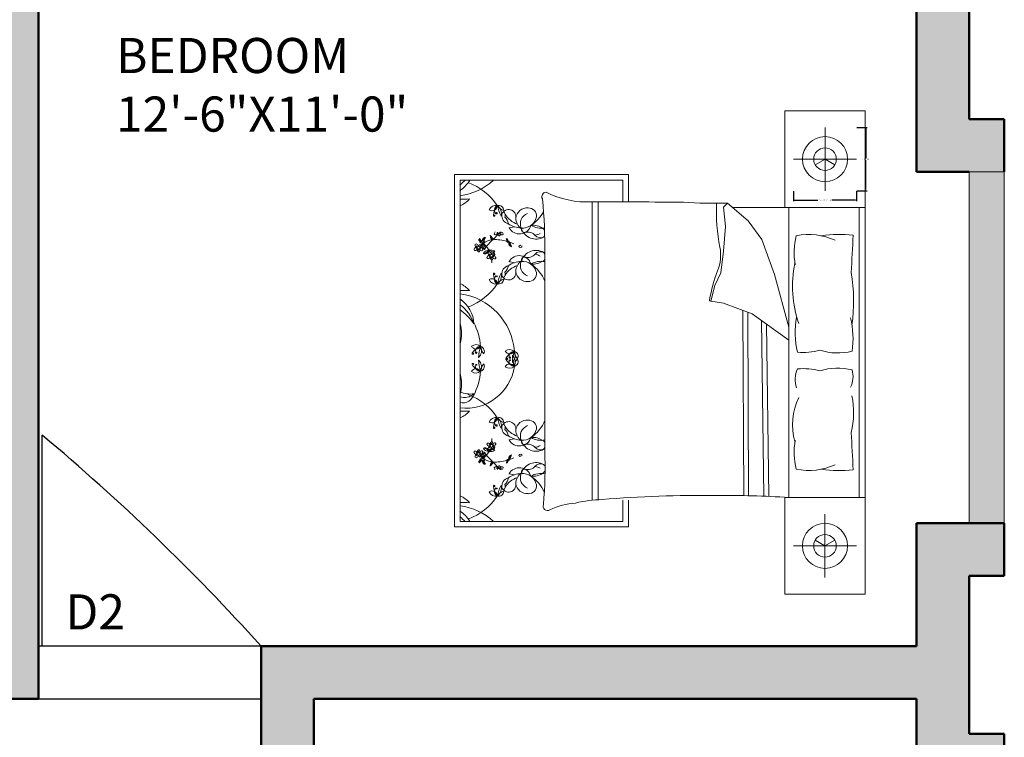
# Model space of a CAD drawing. Units: inches. Extents: x -12 to 604, y -566 to 58.
# Tile 11 of 12: x 436 to 604, y -196 to -74. Entities that reach past the tile are written whole.
import ezdxf

# ---------------------------------------------------------------- set-up
doc = ezdxf.new("R2010")
doc.units = ezdxf.units.IN
doc.header["$MEASUREMENT"] = 0
for name, color, linetype, lineweight in [('A-ANNO-DIMS', 2, 'Continuous', 18), ('A-ANNO-TEXT', 7, 'Continuous', 18), ('A-AREA-IDEN', 7, 'Continuous', 18), ('A-DOOR', 4, 'Continuous', 25), ('A-FURN', 8, 'Continuous', 18), ('A-GLAZ', 82, 'Continuous', 18), ('A-GLAZ-PATT', 82, 'Continuous', 13), ('A-WALL', 7, 'Continuous', 50), ('A-WALL-PATT', 18, 'Continuous', 13)]:
    doc.layers.add(name, color=color, linetype=linetype, lineweight=lineweight)
doc.styles.get("Standard").update_dxf_attribs({"font": 'arial.ttf'})
doc.dimstyles.get("Standard").update_dxf_attribs({"dimtxt": 0.18, "dimasz": 0.18, "dimexe": 0.18, "dimexo": 0.0625, "dimgap": 0.09, "dimtad": 0, "dimtih": 1, "dimtoh": 1, "dimdec": 0, "dimzin": 0, "dimdsep": 46, "dimlunit": 3, "dimtxsty": 'Standard', "dimcen": 0.09, "dimadec": 0, "dimazin": 0, "dimtfac": 1, "dimtdec": 0, "dimtofl": 0, "dimtmove": 0, "dimatfit": 3, "dimfxl": 1, "dimtolj": 1, "dimtzin": 0, "dimarcsym": 0})

# ---------------------------------------------------------------- blocks, each defined once
blk = doc.blocks.new('BEDSIDE-LAMP-196')
for p, q in [((5.39, 10.79), (5.39, 0)), ((0, 5.39), (10.79, 5.39))]:
    blk.add_line(p, q)
for points in [[(5.39, 5.39), (3.72, 6.36)], [(5.39, 5.39), (7.06, 6.36)]]:
    blk.add_lwpolyline(points)
for radius in [3.85, 1.93]:
    blk.add_circle((5.39, 5.39), radius)
blk = doc.blocks.new('*D37')
at = {"layer": 'A-ANNO-DIMS', "color": 0, "lineweight": -2, "transparency": 16777216}
for p, q in [((568.29, -103.17), (568.29, -104.9)), ((579.08, -103.17), (579.08, -104.9)), ((568.47, -104.72), (572.48, -104.72)), ((578.9, -104.72), (574.88, -104.72))]:
    blk.add_line(p, q, dxfattribs=at)
at = {"layer": 'A-ANNO-DIMS', "color": 0, "transparency": 16777216}
for points in [[(568.47, -104.69), (568.47, -104.75), (568.29, -104.72)], [(578.9, -104.69), (578.9, -104.75), (579.08, -104.72)]]:
    blk.add_solid(points, dxfattribs=at)
at = {"layer": 'Defpoints', "color": 0, "transparency": 16777216}
for p in [(568.29, -103.1), (579.08, -103.1), (568.29, -104.72)]:
    blk.add_point(p, dxfattribs=at)
at = {"layer": 'A-ANNO-DIMS', "color": 0, "transparency": 16777216, "insert": (573.68, -104.72), "char_height": 0.18, "attachment_point": 5}
blk.add_mtext('\\A1;LAMP A 0\'-11" TYP.', dxfattribs=at)
blk = doc.blocks.new('*D38')
at = {"layer": 'A-ANNO-DIMS', "color": 0, "lineweight": -2, "transparency": 16777216}
for p, q in [((579.14, -92.32), (580.87, -92.32)), ((580.69, -92.5), (580.69, -97.53)), ((580.69, -102.92), (580.69, -97.89)), ((579.14, -103.1), (580.87, -103.1))]:
    blk.add_line(p, q, dxfattribs=at)
at = {"layer": 'A-ANNO-DIMS', "color": 0, "transparency": 16777216}
for points in [[(580.66, -92.5), (580.72, -92.5), (580.69, -92.32)], [(580.66, -102.92), (580.72, -102.92), (580.69, -103.1)]]:
    blk.add_solid(points, dxfattribs=at)
at = {"layer": 'Defpoints', "color": 0, "transparency": 16777216}
for p in [(579.08, -92.32), (579.08, -103.1), (580.69, -103.1)]:
    blk.add_point(p, dxfattribs=at)
at = {"layer": 'A-ANNO-DIMS', "color": 0, "transparency": 16777216, "insert": (580.69, -97.71), "char_height": 0.18, "attachment_point": 5}
blk.add_mtext('\\A1;0\'-11" TYP.', dxfattribs=at)

msp = doc.modelspace()

# ---------------------------------------------------------------- hatches: boundary and pattern name
at = {"layer": 'A-GLAZ-PATT'}
h = msp.add_hatch(dxfattribs=at)
h.set_pattern_fill('GOST_WOOD', color=256)
h.set_pattern_definition([(90, (0, 0), (6, -4e-16), [10, -2]), (90, (2, -2), (6, -4e-16), [6, -1.5, 3, -1.5]), (90, (4, -5), (6, -4e-16), [10, -2])])
h.paths.add_polyline_path([(344.32, -529.86), (344.32, -520.86), (284.32, -520.86), (284.32, -529.86)])
h.paths.add_polyline_path([(604.32, -450.86), (598.32, -450.86), (598.32, -474.86), (604.32, -474.86)])
h.paths.add_polyline_path([(598.32, -309.28), (604.32, -309.28), (604.32, -274.86), (598.32, -274.86)])
h.paths.add_polyline_path([(598.32, -235.86), (604.32, -235.86), (604.32, -204.86), (598.32, -204.86)])
h.paths.add_polyline_path([(598.32, -159.86), (604.32, -159.86), (604.32, -99.86), (598.32, -99.86)])
at = {"layer": 'A-WALL-PATT'}
h = msp.add_hatch(color=256, dxfattribs=at)
h.dxf.hatch_style = 1
h.paths.add_polyline_path([(169.32, 11.14), (169.32, 17.14), (160.32, 17.14), (160.32, 11.14), (118.32, 11.14), (118.32, 6.64), (118.32, 2.14), (127.32, 2.14), (169.32, 2.14)])
h.paths.add_polyline_path([(127.32, -13.61), (118.32, -13.61), (118.32, -29.36), (34.82, -29.36), (24.32, -29.36), (24.32, -38.36), (39.32, -38.36), (118.32, -38.36), (118.32, -126.86), (127.32, -126.86), (127.32, -117.86)])
h.paths.add_polyline_path([(82.32, -92.36), (39.32, -92.36), (39.32, -56.22), (30.32, -56.22), (24.32, -56.22), (24.32, -65.22), (30.32, -65.22), (30.32, -113.36), (24.32, -113.36), (24.32, -122.36), (39.32, -122.36), (39.32, -101.36), (82.32, -101.36), (82.32, -96.86)], flags=17)
h.paths.add_polyline_path([(280.32, 11.14), (238.32, 11.14), (238.32, 17.14), (229.32, 17.14), (229.32, 12.64), (229.32, 11.14), (229.32, 2.14), (271.32, 2.14), (271.32, -117.86), (163.32, -117.86), (163.32, -126.86), (271.32, -126.86), (271.32, -189.86), (280.32, -189.86), (280.32, -180.86)])
h.paths.add_polyline_path([(415.32, 17.14), (406.32, 17.14), (406.32, 11.14), (358.32, 11.14), (358.32, -21.86), (367.32, -21.86), (367.32, 2.14), (415.32, 2.14)], flags=17)
h.paths.add_polyline_path([(484.55, -45.86), (448.32, -45.86), (448.32, 2.14), (448.32, 17.14), (439.32, 17.14), (439.32, 12.64), (439.32, 2.14), (439.32, -45.86), (367.32, -45.86), (358.32, -45.86), (358.32, -54.86), (430.32, -54.86), (430.32, -69.59), (430.32, -180.86), (318.82, -180.86), (318.82, -189.86), (318.82, -331.86), (327.82, -331.86), (327.82, -189.86), (439.32, -189.86), (439.32, -180.86), (439.32, -54.86), (483.5, -54.86), (484.55, -54.86)])
h.paths.add_polyline_path([(529.32, 11.14), (481.32, 11.14), (481.32, 17.14), (472.32, 17.14), (472.32, 12.64), (472.32, 2.14), (520.32, 2.14), (520.32, -21.86), (529.32, -21.86)])
h.paths.add_polyline_path([(598.32, -45.86), (582.42, -45.86), (582.42, -50.36), (582.42, -54.86), (589.32, -54.86), (589.32, -99.86), (598.32, -99.86), (604.32, -99.86), (604.32, -90.86), (598.32, -90.86)])
h.paths.add_polyline_path([(598.32, -168.86), (604.32, -168.86), (604.32, -159.86), (589.32, -159.86), (589.32, -180.86), (477.32, -180.86), (477.32, -189.86), (477.32, -259.86), (486.32, -259.86), (486.32, -189.86), (589.32, -189.86), (589.32, -204.86), (598.32, -204.86), (604.32, -204.86), (604.32, -195.86), (598.32, -195.86)])
h.paths.add_polyline_path([(598.32, -244.86), (604.32, -244.86), (604.32, -235.86), (598.32, -235.86), (589.32, -235.86), (589.32, -250.86), (522.32, -250.86), (522.32, -259.86), (589.32, -259.86), (589.32, -274.86), (598.32, -274.86), (604.32, -274.86), (604.32, -265.86), (598.32, -265.86)])
h.paths.add_polyline_path([(598.32, -333.28), (604.32, -333.28), (604.32, -324.28), (598.32, -324.28), (598.32, -321.87), (598.32, -318.28), (604.32, -318.28), (604.32, -309.28), (598.32, -309.28), (589.32, -309.28), (589.32, -341.95), (589.38, -341.95), (589.38, -363.16), (589.32, -381.86), (565.32, -381.86), (565.32, -390.86), (589.32, -390.86), (589.32, -450.86), (598.32, -450.86), (604.32, -450.86), (604.32, -441.86), (598.32, -441.86), (598.32, -390.86), (604.32, -390.86), (604.32, -381.86), (598.32, -381.86)])
h.paths.add_polyline_path([(541.32, -345.86), (424.32, -345.86), (424.32, -354.86), (532.32, -354.86), (532.32, -474.86), (463.39, -474.86), (463.39, -483.86), (553.32, -483.86), (553.32, -474.86), (541.32, -474.86), (541.32, -390.86), (541.32, -381.86)])
h.paths.add_polyline_path([(604.32, -474.86), (589.32, -474.86), (553.32, -474.86), (553.32, -483.86), (598.32, -483.86), (604.32, -483.86)])
h.paths.add_polyline_path([(388.32, -483.86), (388.32, -474.86), (388.32, -460.13), (388.32, -333.86), (388.32, -322.86), (379.32, -322.86), (379.32, -331.86), (379.32, -333.86), (379.32, -474.86), (379.32, -520.86), (344.32, -520.86), (344.32, -529.86), (379.32, -529.86), (388.32, -529.86)])
h.paths.add_polyline_path([(284.32, -520.86), (249.32, -520.86), (249.32, -474.86), (249.32, -368.36), (240.32, -368.36), (240.32, -474.86), (238.52, -474.86), (238.52, -483.86), (240.32, -483.86), (240.32, -529.86), (249.32, -529.86), (284.32, -529.86)])
h.paths.add_polyline_path([(178.82, -474.86), (158.91, -474.86), (158.91, -483.86), (162.32, -483.86), (178.82, -483.86)])
h.paths.add_polyline_path([(84.32, -474.86), (84.32, -366.86), (75.32, -366.86), (75.32, -474.86), (39.32, -474.86), (39.32, -453.86), (24.32, -453.86), (24.32, -462.86), (30.32, -462.86), (30.32, -483.86), (84.32, -483.86)])
h.paths.add_polyline_path([(39.32, -342.86), (75.32, -342.86), (84.32, -342.86), (179.67, -342.86), (179.67, -333.86), (39.32, -333.86), (39.32, -318.86), (24.32, -318.86), (24.32, -327.86), (30.32, -327.86), (30.32, -432.86), (24.32, -432.86), (24.32, -441.86), (30.32, -441.86), (39.32, -441.86)])
h.paths.add_polyline_path([(249.32, -252.86), (115.32, -252.86), (115.32, -225.86), (106.32, -225.86), (106.32, -252.86), (39.32, -252.86), (39.32, -237.86), (24.32, -237.86), (24.32, -246.86), (30.32, -246.86), (30.32, -267.86), (24.32, -267.86), (24.32, -276.86), (39.32, -276.86), (39.32, -261.86), (240.32, -261.86), (240.32, -331.86), (249.32, -331.86), (266.82, -331.86), (266.82, -322.86), (249.32, -322.86)])
h.paths.add_polyline_path([(127.32, -180.86), (39.32, -180.86), (24.32, -180.86), (24.32, -189.86), (39.32, -189.86), (127.32, -189.86)])
h.paths.add_polyline_path([(39.32, -159.86), (24.32, -159.86), (24.32, -168.86), (30.32, -168.86), (30.32, -180.86), (39.32, -180.86)])
h.paths.add_polyline_path([(470.51, -17.27), (512.48, -17.27), (512.48, 5.12), (470.51, 5.12)], flags=9)
h.paths.add_polyline_path([(484.21, -244.26), (526.45, -244.26), (526.45, -221.87), (484.21, -221.87)], flags=24)
h.paths.add_polyline_path([(36.91, -442.88), (83.54, -442.88), (83.54, -420.5), (36.91, -420.5)], flags=25)

# ---------------------------------------------------------------- linework, layer by layer
at = {"layer": 'A-DOOR'}
for p, q in [((439.95, -180.86), (439.95, -144.86)), ((477.32, -180.86), (439.32, -180.86)), ((439.32, -180.86), (439.32, -189.86)), ((477.32, -189.86), (477.32, -180.86)), ((439.32, -189.86), (477.32, -189.86))]:
    msp.add_line(p, q, dxfattribs=at)
msp.add_arc((202.75, -428.5), 369.75, 42.0482, 50.0958, dxfattribs=at)
at = {"layer": 'A-FURN'}
for p, q in [((580.56, -89.46), (580.56, -172)), ((510.36, -100.35), (540.1, -100.35)), ((510.36, -160.53), (510.36, -100.35)), ((540.1, -100.35), (540.1, -105.02)), ((511.32, -101.31), (511.32, -159.57)), ((539.14, -101.31), (511.32, -101.31)), ((539.14, -105.02), (539.14, -101.31)), ((533.92, -155.95), (533.92, -105.01)), ((534.95, -155.87), (534.95, -105.01)), ((556.37, -105.9), (557.04, -105.23)), ((556.71, -109.24), (556.37, -105.9)), ((557.04, -105.23), (560.55, -108.24)), ((580.56, -105.97), (557.9, -105.97)), ((567.52, -105.97), (567.52, -155.49)), ((579.5, -155.49), (579.5, -105.97)), ((519.69, -109.44), (520.62, -109.26)), ((556.37, -113.42), (556.71, -109.24)), ((560.55, -108.24), (562.89, -111.41)), ((562.89, -111.41), (565.06, -117.43)), ((525.81, -147.49), (525.81, -113.97)), ((555.87, -117.1), (556.37, -113.42)), ((519.69, -115.21), (520.62, -115.39)), ((554.87, -119.27), (555.87, -117.1)), ((565.06, -117.43), (567.52, -126.43)), ((554.2, -121.95), (554.87, -119.27)), ((556.37, -122.28), (554.2, -121.95)), ((561.22, -124.12), (556.37, -122.28)), ((559.79, -155.2), (559.66, -123.53)), ((560.64, -155.2), (560.52, -123.85)), ((567.52, -128.64), (561.22, -124.12)), ((563.24, -155.24), (562.82, -125.27)), ((564.09, -155.27), (563.68, -125.88)), ((519.69, -145.67), (520.62, -145.49)), ((519.69, -151.44), (520.62, -151.62)), ((539.14, -159.57), (539.14, -155.94)), ((540.1, -155.95), (540.1, -160.53)), ((511.32, -159.57), (539.14, -159.57)), ((540.1, -160.53), (510.36, -160.53))]:
    msp.add_line(p, q, dxfattribs=at)
for points in [[(566.8, -105.97), (566.8, -89.46), (580.56, -89.46)], [(580.56, -155.49), (566.8, -155.49), (566.8, -172), (580.56, -172)]]:
    msp.add_lwpolyline(points, dxfattribs=at)
for points in [[(549.48, -105.05, 0.001242), (533.82, -105.01, -0.127202), (526.02, -103.36)], [(578.5, -110.71, 0.074897), (573.11, -110.81, -0.472817)], [(572.81, -130.34, 0.14099), (578.31, -130.51, 0.235245)], [(572.81, -133.87, -0.14099), (578.31, -133.7, -0.235245)], [(578.5, -150.75, -0.074897), (573.11, -150.65, 0.472817)], [(535.6, -155.85, 0.056112), (531.06, -156.44, 0.095341), (526.68, -157.6)]]:
    msp.add_lwpolyline(points, format="xyb", dxfattribs=at)
for centre in [(514.48, -112.84), (516.7, -114.21), (514.48, -148.05), (516.7, -146.67)]:
    msp.add_circle(centre, 0.21, dxfattribs=at)
for centre, radius, start, end in [((507.44, -96.8), 6.55, 306.3036, 316.4814), ((508.42, -98.69), 5.25, 303.4617, 330.1116), ((509.87, -93.28), 10.78, 277.745, 311.8856), ((508.8, -111.73), 10.78, 34.3865, 68.5908), ((526.07, -104.12), 0.762, 93.98, 207.3412), ((509.64, -101.63), 4.38, 292.5547, 318.9546), ((511.99, -89.63), 14.91, 267.4081, 273.6519), ((517.44, -106.81), 1.2, 77.7115, 159.0387), ((516.8, -105.61), 0.9, 238.4633, 358.2869), ((519.75, -107.43), 2.73, 138.8402, 177.9352), ((518.1, -106.42), 0.882, 117.6827, 223.7762), ((517.91, -106.51), 0.894, 2.9516, 103.728), ((525.06, -104), 7.54, 192.5173, 207.1824), ((516.7, -107.02), 1.7, 345.4653, 54.2343), ((519.27, -104.68), 1.84, 211.3827, 255.2969), ((439.89, -112.99), 85.93, 359.3433, 5.6887), ((554.99, -29.54), 75.71, 265.8294, 271.553), ((586.27, -106.64), 31.15, 177.4519, 191.3392), ((517.16, -107.34), 0.134, 177.9352, 11.4834), ((517.22, -107.32), 0.065, 11.4834, 127.9409), ((517.55, -106.95), 0.117, 223.7762, 159.7183), ((519.62, -107.55), 1.24, 350.264, 160.8688), ((519.99, -107.26), 1.55, 175.969, 254.3045), ((518.28, -107.3), 0.759, 333.9755, 53.2681), ((517.94, -108.92), 1.65, 6.1662, 51.5825), ((522.35, -105.1), 3.9, 211.2614, 251.7045), ((522.8, -108.01), 1.97, 84.9449, 172.8857), ((523.55, -108.78), 1.92, 111.5819, 201.4221), ((521.97, -107.01), 2.48, 265.2933, 346.921), ((523, -107.44), 1.39, 354.4856, 91.0538), ((520, -103.8), 6.25, 303.6671, 333.2997), ((522.03, -105.06), 4.43, 236.2883, 266.5076), ((521.47, -108.42), 2.05, 209.9085, 343.1337), ((523.24, -107.67), 2.4, 182.3591, 234.0401), ((525.2, -106.09), 3.42, 238.8218, 279.1554), ((523.71, -112.17), 3.18, 55.785, 94.7304), ((518.83, -110.84), 2.33, 178.3264, 187.1302), ((516.31, -111.16), 0.433, 11.3256, 64.4621), ((517.78, -110.54), 1.3, 190.2588, 210.656), ((511.58, -105.75), 7.84, 313.1541, 322.0459), ((517.34, -110.46), 0.161, 142.4737, 265.053), ((517.56, -110.42), 0.347, 127.7621, 169.0403), ((517.37, -110.13), 0.489, 265.053, 338.3618), ((518.02, -110.8), 0.638, 113.4276, 137.6104), ((517.94, -110.14), 0.21, 183.2768, 356.7232), ((518.1, -110.52), 0.344, 139.7889, 227.6792), ((517.99, -110.64), 0.181, 227.6792, 350.3487), ((517.29, -110.51), 0.688, 353.0852, 15.7171), ((517.74, -110.59), 0.435, 350.3487, 43.6538), ((518.55, -110.15), 0.506, 198.7263, 262.5032), ((518.14, -110.38), 0.201, 1.1081, 91.8675), ((518.27, -110.43), 0.351, 11.5637, 52.6358), ((518.52, -110.49), 0.162, 255.2356, 54.9248), ((522.33, -109.72), 0.512, 167.3041, 285.1471), ((523.71, -112.17), 3.18, 122.7011, 126.3445), ((524.31, -108.74), 2.63, 199.2822, 299.1751), ((522.9, -111.85), 1.69, 41.5653, 105.1471), ((523.84, -108.34), 2.37, 277.436, 299.9149), ((525.09, -109.9), 1.24, 221.5653, 293.8354), ((524.9, -110.33), 0.994, 30.0293, 52.325), ((524.9, -110.33), 0.994, 314.4517, 333.558), ((579.47, -113.65), 11.06, 165.1039, 191.0369), ((570.95, -121.22), 10.64, 65.1316, 101.7583), ((1364.07, -156.21), 786.88, 176.68521, 177.14978), ((514.32, -112.41), 0.415, 157.4086, 261.4386), ((514.09, -112.4), 0.208, 58.0499, 135.6268), ((514.3, -112.53), 0.139, 172.906, 277.132), ((513.84, -112.78), 0.663, 14.7558, 58.0499), ((514.77, -112.6), 0.287, 36.1046, 181.4281), ((514.79, -111.48), 0.235, 124.3538, 214.3923), ((515.13, -111.52), 0.547, 190.3057, 287.1958), ((514.61, -112.38), 0.289, 270.0645, 331.1507), ((514.85, -112.45), 0.331, 221.8413, 265.7877), ((515.29, -111.32), 0.635, 176.9701, 248.2913), ((519.82, -107.97), 6.14, 212.6784, 216.3746), ((514.85, -112.57), 0.206, 263.7526, 41.7054), ((515.07, -111.47), 0.243, 216.3746, 291.7548), ((517.22, -114.88), 3.43, 124.0033, 132.4917), ((513.7, -115.31), 3.66, 63.7819, 68.2913), ((515.65, -112.5), 0.582, 128.3208, 208.8162), ((515.65, -111.64), 0.547, 122.8155, 187.3992), ((515.23, -111.87), 0.183, 289.3605, 111.7548), ((515.37, -111.87), 0.183, 221.8703, 44.2646), ((516.2, -112.4), 0.958, 157.2305, 229.0635), ((515.89, -111.71), 0.635, 109.4799, 177.6828), ((515.88, -112.08), 0.564, 174.4544, 220.6188), ((512.67, -115.23), 4.11, 30.544, 49.818), ((515.55, -111.31), 0.235, 56.8636, 146.9021), ((515.67, -111.57), 0.243, 148.8844, 224.2646), ((514.94, -112.89), 0.678, 340.0041, 40.6188), ((520.72, -114.62), 6.14, 145.1882, 148.8844), ((517.22, -114.88), 3.43, 94.756, 119.2041), ((524.52, -119.81), 11.28, 132.2412, 142.1744), ((516.91, -111.07), 0.396, 188.3432, 274.2869), ((517.26, -110.85), 0.692, 210.656, 242.6341), ((517.78, -110.26), 1.33, 218.2101, 226.3071), ((516.8, -111.37), 0.168, 325.7657, 67.4417), ((517.4, -118.29), 6.84, 73.5842, 93.8277), ((521.61, -111.33), 2.33, 178.3264, 187.1302), ((519.09, -111.65), 0.433, 11.3256, 64.4621), ((520.56, -111.03), 1.3, 190.2588, 210.656), ((519.69, -111.56), 0.396, 188.3432, 274.2869), ((520.04, -111.34), 0.692, 210.656, 242.6341), ((520.56, -110.75), 1.33, 218.2101, 226.3071), ((519.58, -111.86), 0.168, 325.7657, 67.4417), ((520.05, -112.17), 0.396, 147.5332, 233.4768), ((520.41, -111.97), 0.692, 179.1859, 211.164), ((519.74, -112.12), 0.168, 354.3784, 96.0543), ((517.4, -118.29), 6.84, 63.0032, 69.8941), ((520.93, -111.65), 1.3, 211.164, 231.5612), ((521.16, -110.59), 2.33, 234.6898, 243.4936), ((521.18, -111.79), 1.33, 195.5129, 203.6099), ((519.69, -112.65), 0.433, 357.3579, 50.4944), ((521.55, -112.56), 0.159, 12.7051, 190.4384), ((521.65, -112.55), 0.259, 190.4384, 10.4136), ((513.88, -113.16), 0.161, 142.4737, 265.053), ((514.09, -113.12), 0.347, 61.2196, 169.0403), ((513.91, -112.83), 0.489, 265.053, 338.3618), ((514.55, -113.5), 0.638, 113.4276, 137.6104), ((514.63, -113.22), 0.344, 139.7889, 227.6792), ((514.52, -113.34), 0.181, 227.6792, 350.3487), ((513.82, -113.21), 0.688, 353.0852, 15.7171), ((514.27, -113.3), 0.435, 350.3487, 43.6538), ((515.08, -112.85), 0.506, 198.7263, 262.5032), ((514.68, -113.08), 0.201, 1.1081, 91.8675), ((514.81, -113.13), 0.351, 11.5637, 86.365), ((515.06, -113.19), 0.162, 255.2356, 54.9248), ((515.76, -112.45), 0.696, 207.7043, 254.3516), ((515.31, -112.85), 0.958, 270.278, 342.111), ((515.95, -114.05), 0.678, 98.7227, 159.3375), ((515.61, -113.18), 0.696, 244.9899, 291.6373), ((515.76, -112.82), 0.564, 278.7227, 324.8872), ((515.66, -113.28), 0.582, 290.5253, 358.5375), ((516.31, -114.5), 0.347, 61.2196, 169.0403), ((516.12, -114.2), 0.489, 265.053, 338.3618), ((516.54, -113.78), 0.415, 157.4086, 261.4386), ((516.3, -113.77), 0.208, 58.0499, 135.6268), ((516.79, -113.11), 0.582, 182.8499, 266.1226), ((516.57, -112.7), 0.564, 231.7607, 277.9252), ((517.01, -112.6), 0.958, 214.5369, 286.3699), ((516.77, -114.87), 0.638, 113.4276, 137.6104), ((516.52, -113.9), 0.139, 172.906, 277.132), ((516.06, -114.16), 0.663, 14.7558, 58.0499), ((512.67, -115.23), 4.11, 23.0501, 23.8477), ((516.85, -114.59), 0.344, 139.7889, 227.6792), ((516.74, -113.93), 0.678, 37.3105, 97.9252), ((516.99, -113.98), 0.287, 36.1046, 181.4281), ((516.04, -114.59), 0.688, 353.0852, 15.7171), ((516.82, -113), 0.696, 265.0106, 311.658), ((516.49, -114.67), 0.435, 350.3487, 43.6538), ((516.82, -113.75), 0.289, 270.0645, 331.1507), ((517.07, -113.82), 0.331, 221.8413, 265.7877), ((517.3, -114.22), 0.506, 198.7263, 262.5032), ((516.89, -114.46), 0.201, 1.1081, 91.8675), ((517.07, -113.95), 0.206, 263.7526, 41.7054), ((517.02, -114.5), 0.351, 11.5637, 86.365), ((521.47, -116.24), 2.05, 16.8663, 150.0915), ((524.31, -115.92), 2.63, 60.8249, 160.7178), ((522.9, -112.81), 1.69, 254.8529, 318.4347), ((523.84, -116.31), 2.37, 60.0851, 82.564), ((525.09, -114.75), 1.24, 66.1646, 138.4347), ((524.9, -114.33), 0.994, 23.229, 45.5483), ((549.14, -114.09), 6.72, 336.2616, 11.3392), ((516.09, -114.53), 0.161, 142.4737, 265.053), ((516.74, -114.71), 0.181, 227.6792, 350.3487), ((512.67, -115.23), 4.11, 357.1071, 4.7585), ((517.27, -114.57), 0.162, 255.2356, 54.9248), ((519.99, -117.4), 1.55, 105.6955, 184.031), ((517.94, -115.73), 1.65, 308.4175, 353.8338), ((522.35, -119.56), 3.9, 108.2955, 148.7386), ((522.03, -119.59), 4.43, 93.4924, 123.7117), ((523.24, -116.99), 2.4, 125.9599, 177.6409), ((523.55, -115.87), 1.92, 158.5779, 248.4181), ((521.97, -117.65), 2.48, 13.079, 94.7067), ((522.33, -114.94), 0.512, 74.8529, 192.6959), ((523.71, -112.48), 3.18, 233.6555, 237.2989), ((525.2, -118.57), 3.42, 79.7133, 121.1782), ((523.71, -112.48), 3.18, 265.2696, 304.215), ((520, -120.86), 6.25, 21.4941, 56.3329), ((524.9, -114.33), 0.994, 307.675, 336.7144), ((587.33, -119.47), 19.19, 168.0397, 199.2615), ((517.16, -117.32), 0.134, 348.5166, 182.0648), ((519.75, -117.22), 2.73, 182.0648, 221.1598), ((517.22, -117.33), 0.065, 232.0591, 348.5166), ((518.1, -118.24), 0.882, 136.2238, 242.3173), ((517.6, -117.72), 0.0703, 200.2667, 136.2271), ((516.7, -117.63), 1.7, 305.7657, 14.5347), ((525.06, -120.65), 7.54, 152.8176, 167.4827), ((519.62, -117.1), 1.24, 199.1312, 9.736), ((518.28, -117.35), 0.759, 306.7319, 26.0245), ((522.8, -116.65), 1.97, 187.1143, 275.0551), ((523, -117.22), 1.39, 268.9462, 5.5144), ((585.4, -127.68), 32.01, 160.1194, 169.3383), ((548.63, -122.02), 29.94, 352.2196, 9.497), ((509.64, -123.02), 4.38, 41.0454, 67.4453), ((508.8, -112.93), 10.78, 291.4092, 325.6135), ((516.8, -119.04), 0.9, 1.7131, 121.5367), ((517.44, -117.85), 1.2, 200.9613, 282.2885), ((517.91, -118.15), 0.894, 256.272, 357.0484), ((519.27, -119.98), 1.84, 104.7031, 148.6173), ((511.99, -135.03), 14.91, 86.3481, 92.5919), ((509.87, -131.37), 10.78, 4.4623, 82.255), ((508.42, -125.96), 5.25, 1.272, 56.5383), ((507.44, -127.85), 6.55, 17.8504, 53.6964), ((554.14, -121.76), 0.199, 178.8623, 289.7536), ((505.6, -131.29), 9.74, 34.0123, 54.053), ((505.65, -127.53), 5.93, 343.5431, 17.0202), ((504.09, -130.55), 10.78, 4.4623, 27.4146), ((583.14, -127.24), 14.56, 169.8617, 193.6238), ((563.76, -128.34), 14.71, 351.5249, 13.96), ((502.6, -129.88), 8.76, 4.3787, 5.6357), ((496.59, -134.5), 15.66, 19.7217, 19.9028), ((514.04, -130.59), 1.2, 47.7873, 129.1145), ((514.07, -129.24), 0.9, 208.5391, 328.3627), ((513.52, -130.91), 0.134, 148.011, 341.5592), ((515.72, -132.29), 2.73, 108.9159, 148.011), ((513.59, -130.93), 0.065, 341.5592, 98.0167), ((514.8, -130.59), 0.882, 87.7585, 193.852), ((514.06, -130.77), 0.117, 193.852, 129.9245), ((522.03, -131.96), 7.54, 162.593, 177.2582), ((513.29, -130.41), 1.7, 315.5411, 24.3101), ((516.68, -129.66), 1.84, 181.4585, 225.3727), ((514.59, -130.57), 0.894, 333.0274, 73.8037), ((519.81, -131.42), 1.2, 47.7873, 129.1145), ((519.85, -130.06), 0.9, 208.5391, 328.3627), ((521.5, -133.11), 2.73, 108.9159, 148.011), ((520.58, -131.41), 0.882, 87.7585, 193.852), ((519.06, -131.23), 1.7, 315.5411, 24.3101), ((527.81, -132.79), 7.54, 162.593, 177.2582), ((519.06, -132.4), 1.7, 335.6899, 44.4589), ((527.81, -130.85), 7.54, 182.7418, 197.407), ((520.36, -131.39), 0.894, 333.0274, 73.8037), ((522.45, -130.49), 1.84, 181.4585, 225.3727), ((570.05, -120.61), 10.11, 264.0129, 285.8293), ((513.52, -132.72), 0.134, 18.4408, 211.989), ((515.72, -131.35), 2.73, 211.989, 251.0841), ((513.59, -132.7), 0.065, 261.9833, 18.4408), ((514.8, -133.05), 0.882, 166.148, 272.2415), ((514.11, -132.85), 0.0703, 230.1909, 166.0209), ((522.03, -131.67), 7.54, 182.7418, 197.407), ((513.29, -133.23), 1.7, 335.6899, 44.4589), ((516.68, -133.97), 1.84, 134.6273, 178.5415), ((514.59, -133.07), 0.894, 286.1963, 26.9726), ((519.85, -133.57), 0.9, 31.6373, 151.4609), ((519.3, -131.74), 0.134, 148.011, 341.5592), ((519.3, -131.9), 0.134, 18.4408, 211.989), ((521.5, -130.52), 2.73, 211.989, 251.0841), ((519.36, -131.76), 0.065, 341.5592, 98.0167), ((519.36, -131.87), 0.065, 261.9833, 18.4408), ((520.58, -132.22), 0.882, 166.148, 272.2415), ((519.83, -131.6), 0.117, 193.852, 129.9245), ((519.88, -132.03), 0.0703, 230.1909, 166.0209), ((520.36, -132.24), 0.894, 286.1963, 26.9726), ((522.45, -133.15), 1.84, 134.6273, 178.5415), ((512.35, -131.91), 8.34, 262.8636, 351.8197), ((505.65, -136.1), 5.93, 342.9798, 16.4569), ((502.6, -133.75), 8.76, 354.3643, 355.6213), ((496.59, -129.14), 15.66, 340.0972, 340.2783), ((514.07, -134.4), 0.9, 31.6373, 151.4609), ((514.04, -133.04), 1.2, 230.8855, 312.2127), ((504.09, -133.09), 10.78, 332.5854, 355.5377), ((519.81, -132.22), 1.2, 230.8855, 312.2127), ((572.96, -135.39), 4.38, 155.0183, 198.5407), ((570.05, -143.6), 10.11, 74.1707, 95.9871), ((574.39, -134.84), 4.08, 333.3437, 16.1026), ((513.12, -132.99), 4.83, 248.117, 276.6195), ((511.77, -137.42), 1.93, 256.3898, 349.0739), ((512.04, -135.97), 2.45, 252.8609, 311.9049), ((508.8, -147.95), 10.78, 34.3865, 68.5908), ((578.65, -143.03), 10.51, 153.8761, 196.1746), ((564.06, -140.95), 14.51, 346.3427, 11.1841), ((511.99, -125.86), 14.91, 267.4081, 273.6519), ((509.64, -137.86), 4.38, 292.5547, 318.9546), ((517.44, -143.03), 1.2, 77.7115, 159.0387), ((516.8, -141.84), 0.9, 238.4633, 358.2869), ((519.75, -143.66), 2.73, 138.8402, 177.9352), ((518.1, -142.65), 0.882, 117.6827, 223.7762), ((517.91, -142.73), 0.894, 2.9516, 103.728), ((519.27, -140.91), 1.84, 211.3827, 255.2969), ((516.7, -143.25), 1.7, 345.4653, 54.2343), ((525.06, -140.23), 7.54, 192.5173, 207.1824), ((519.62, -143.78), 1.24, 350.264, 160.8688), ((518.28, -143.53), 0.759, 333.9755, 53.2681), ((522.8, -144.24), 1.97, 84.9449, 172.8857), ((523, -143.67), 1.39, 354.4856, 91.0538), ((520, -140.03), 6.25, 303.6671, 338.5059), ((517.16, -143.57), 0.134, 177.9352, 11.4834), ((517.22, -143.55), 0.065, 11.4834, 127.9409), ((517.55, -143.18), 0.117, 223.7762, 159.7183), ((519.99, -143.49), 1.55, 175.969, 254.3045), ((517.94, -145.15), 1.65, 6.1662, 51.5825), ((522.35, -141.33), 3.9, 211.2614, 251.7045), ((523.24, -143.89), 2.4, 182.3591, 234.0401), ((523.55, -145.01), 1.92, 111.5819, 201.4221), ((521.97, -143.24), 2.48, 265.2933, 346.921), ((1364.07, -105.25), 786.88, 182.85022, 183.31479), ((516.09, -146.35), 0.161, 94.947, 217.5263), ((516.12, -146.68), 0.489, 21.6382, 94.947), ((516.85, -146.29), 0.344, 132.3208, 220.2111), ((516.74, -146.17), 0.181, 9.6513, 132.3208), ((516.04, -146.3), 0.688, 344.2829, 6.9148), ((512.67, -145.65), 4.11, 355.2415, 2.8929), ((516.49, -146.21), 0.435, 316.3462, 9.6513), ((517.3, -146.66), 0.506, 97.4968, 161.2737), ((517.27, -146.32), 0.162, 305.0752, 104.7644), ((522.03, -141.29), 4.43, 236.2883, 266.5076), ((521.47, -144.65), 2.05, 209.9085, 343.1337), ((522.33, -145.95), 0.512, 167.3041, 285.1471), ((523.71, -148.4), 3.18, 122.7011, 126.3445), ((524.31, -144.97), 2.63, 199.2822, 299.1751), ((525.2, -142.32), 3.42, 238.8218, 280.2867), ((523.71, -148.4), 3.18, 55.785, 94.7304), ((524.9, -146.55), 0.994, 23.2856, 52.325), ((579.47, -147.81), 11.06, 168.9631, 194.8961), ((513.88, -147.73), 0.161, 94.947, 217.5263), ((514.09, -147.76), 0.347, 190.9597, 298.7804), ((513.91, -148.05), 0.489, 21.6382, 94.947), ((514.55, -147.39), 0.638, 222.3896, 246.5724), ((514.63, -147.67), 0.344, 132.3208, 220.2111), ((514.52, -147.55), 0.181, 9.6513, 132.3208), ((513.82, -147.67), 0.688, 344.2829, 6.9148), ((514.27, -147.59), 0.435, 316.3462, 9.6513), ((515.08, -148.04), 0.506, 97.4968, 161.2737), ((514.68, -147.8), 0.201, 268.1325, 358.8919), ((514.81, -147.76), 0.351, 273.635, 348.4363), ((515.06, -147.69), 0.162, 305.0752, 104.7644), ((515.76, -148.43), 0.696, 105.6484, 152.2957), ((516.2, -148.48), 0.958, 130.9365, 202.7695), ((515.61, -147.7), 0.696, 68.3627, 115.0101), ((515.31, -148.03), 0.958, 17.889, 89.722), ((515.95, -146.83), 0.678, 200.6625, 261.2773), ((512.67, -145.65), 4.11, 310.182, 329.456), ((514.94, -147.99), 0.678, 319.3812, 19.9959), ((524.52, -141.07), 11.28, 217.8256, 227.7588), ((515.76, -148.06), 0.564, 35.1128, 81.2773), ((515.66, -147.6), 0.582, 1.4625, 69.4747), ((516.31, -146.38), 0.347, 190.9597, 298.7804), ((516.54, -147.1), 0.415, 98.5614, 202.5914), ((516.3, -147.11), 0.208, 224.3732, 301.9501), ((516.79, -147.77), 0.582, 93.8774, 177.1501), ((517.01, -148.28), 0.958, 73.6301, 145.4631), ((516.57, -148.18), 0.564, 82.0748, 128.2393), ((516.77, -146.01), 0.638, 222.3896, 246.5724), ((516.52, -146.98), 0.139, 82.868, 187.094), ((516.06, -146.73), 0.663, 301.9501, 345.2442), ((512.67, -145.65), 4.11, 336.1523, 336.9499), ((516.74, -146.95), 0.678, 262.0748, 322.6895), ((516.99, -146.9), 0.287, 178.5719, 323.8954), ((516.82, -147.88), 0.696, 48.342, 94.9894), ((517.07, -147.06), 0.331, 94.2123, 138.1587), ((516.82, -147.13), 0.289, 28.8493, 89.9355), ((516.89, -146.43), 0.201, 268.1325, 358.8919), ((517.02, -146.38), 0.351, 273.635, 348.4363), ((517.07, -146.94), 0.206, 318.2946, 96.2474), ((522.9, -148.08), 1.69, 41.5653, 105.1471), ((523.84, -144.57), 2.37, 277.436, 299.9149), ((525.09, -146.13), 1.24, 221.5653, 293.8354), ((445.53, -150.01), 80.32, 355.2402, 1.8035), ((524.9, -146.55), 0.994, 314.4517, 336.7144), ((514.32, -148.47), 0.415, 98.5614, 202.5914), ((514.09, -148.49), 0.208, 224.3732, 301.9501), ((514.3, -148.36), 0.139, 82.868, 187.094), ((513.84, -148.1), 0.663, 301.9501, 345.2442), ((514.77, -148.28), 0.287, 178.5719, 323.8954), ((514.79, -149.4), 0.235, 145.6077, 235.6462), ((515.13, -149.37), 0.547, 72.8042, 169.6943), ((514.85, -148.44), 0.331, 94.2123, 138.1587), ((514.61, -148.5), 0.289, 28.8493, 89.9355), ((515.29, -149.56), 0.635, 111.7087, 183.0299), ((519.82, -152.91), 6.14, 143.6254, 147.3216), ((514.85, -148.31), 0.206, 318.2946, 96.2474), ((515.07, -149.41), 0.243, 68.2452, 143.6254), ((517.22, -146), 3.43, 227.5083, 235.9967), ((513.7, -145.57), 3.66, 291.7087, 296.2181), ((515.65, -148.39), 0.582, 151.1838, 231.6792), ((515.65, -149.24), 0.547, 172.6008, 237.1845), ((515.23, -149.02), 0.183, 248.2452, 70.6395), ((515.37, -149.02), 0.183, 315.7354, 138.1297), ((515.89, -149.17), 0.635, 182.3172, 250.5201), ((515.88, -148.8), 0.564, 139.3812, 185.5456), ((515.55, -149.58), 0.235, 213.0979, 303.1364), ((515.67, -149.31), 0.243, 135.7354, 211.1156), ((520.72, -146.27), 6.14, 211.1156, 214.8118), ((517.22, -146), 3.43, 240.7959, 265.244), ((517.78, -150.35), 1.3, 149.344, 169.7412), ((516.91, -149.81), 0.396, 85.7131, 171.6568), ((517.26, -150.03), 0.692, 117.3659, 149.344), ((517.78, -150.63), 1.33, 133.6929, 141.7899), ((516.8, -149.51), 0.168, 292.5583, 34.2343), ((517.4, -142.6), 6.84, 266.1723, 286.4158), ((511.58, -155.14), 7.84, 37.9541, 46.8459), ((520.56, -149.85), 1.3, 149.344, 169.7412), ((521.61, -149.55), 2.33, 172.8698, 181.6736), ((519.09, -149.23), 0.433, 295.5379, 348.6744), ((519.69, -149.32), 0.396, 85.7131, 171.6568), ((520.04, -149.54), 0.692, 117.3659, 149.344), ((520.56, -150.14), 1.33, 133.6929, 141.7899), ((519.58, -149.02), 0.168, 292.5583, 34.2343), ((520.05, -148.71), 0.396, 126.5232, 212.4668), ((520.41, -148.92), 0.692, 148.836, 180.8141), ((519.74, -148.76), 0.168, 263.9457, 5.6216), ((517.4, -142.6), 6.84, 290.1059, 296.9968), ((520.93, -149.23), 1.3, 128.4388, 148.836), ((521.16, -150.3), 2.33, 116.5064, 125.3102), ((521.18, -149.1), 1.33, 156.3901, 164.4871), ((519.69, -148.23), 0.433, 309.5056, 2.6421), ((521.65, -148.34), 0.259, 349.5864, 169.5616), ((521.55, -148.32), 0.159, 169.5616, 347.2949), ((524.31, -152.15), 2.63, 60.8249, 160.7178), ((518.83, -150.05), 2.33, 172.8698, 181.6736), ((516.31, -149.72), 0.433, 295.5379, 348.6744), ((517.34, -150.43), 0.161, 94.947, 217.5263), ((517.56, -150.46), 0.347, 190.9597, 232.2379), ((517.37, -150.75), 0.489, 21.6382, 94.947), ((518.02, -150.09), 0.638, 222.3896, 246.5724), ((517.94, -150.75), 0.21, 3.2768, 176.7232), ((518.1, -150.37), 0.344, 132.3208, 220.2111), ((517.99, -150.25), 0.181, 9.6513, 132.3208), ((517.29, -150.37), 0.688, 344.2829, 6.9148), ((517.74, -150.29), 0.435, 316.3462, 9.6513), ((518.55, -150.74), 0.506, 97.4968, 161.2737), ((518.14, -150.5), 0.201, 268.1325, 358.8919), ((518.52, -150.39), 0.162, 305.0752, 104.7644), ((518.27, -150.46), 0.351, 307.3642, 348.4363), ((522.03, -155.82), 4.43, 93.4924, 123.7117), ((521.47, -152.46), 2.05, 16.8663, 150.0915), ((523.24, -153.22), 2.4, 125.9599, 177.6409), ((523.55, -152.1), 1.92, 158.5779, 248.4181), ((521.97, -153.87), 2.48, 13.079, 94.7067), ((522.33, -151.16), 0.512, 74.8529, 192.6959), ((523.71, -148.71), 3.18, 233.6555, 237.2989), ((522.9, -149.04), 1.69, 254.8529, 318.4347), ((525.2, -154.79), 3.42, 79.249, 121.1782), ((523.71, -148.71), 3.18, 265.2696, 304.215), ((523.84, -152.54), 2.37, 60.0851, 82.564), ((525.09, -150.98), 1.24, 66.1646, 138.4347), ((524.9, -150.56), 0.994, 307.675, 342.5814), ((524.9, -150.56), 0.994, 16.6343, 45.5483), ((570.95, -140.24), 10.64, 258.2417, 294.8684), ((519.99, -153.63), 1.55, 105.6955, 184.031), ((517.94, -151.96), 1.65, 308.4175, 353.8338), ((522.35, -155.78), 3.9, 108.2955, 148.7386), ((520, -157.09), 6.25, 23.6453, 56.3329), ((516.8, -155.27), 0.9, 1.7131, 121.5367), ((517.44, -154.08), 1.2, 200.9613, 282.2885), ((517.16, -153.54), 0.134, 348.5166, 182.0648), ((519.75, -153.45), 2.73, 182.0648, 221.1598), ((517.22, -153.56), 0.065, 232.0591, 348.5166), ((518.1, -154.46), 0.882, 136.2238, 242.3173), ((517.6, -153.95), 0.0703, 200.2667, 136.2271), ((525.06, -156.88), 7.54, 152.8176, 167.4827), ((516.7, -153.86), 1.7, 305.7657, 14.5347), ((519.27, -156.2), 1.84, 104.7031, 148.6173), ((517.91, -154.38), 0.894, 256.272, 357.0484), ((519.62, -153.33), 1.24, 199.1312, 9.736), ((518.28, -153.58), 0.759, 306.7319, 26.0245), ((522.8, -152.87), 1.97, 187.1143, 275.0551), ((523, -153.45), 1.39, 268.9462, 5.5144), ((509.64, -159.25), 4.38, 41.0454, 67.4453), ((511.99, -171.26), 14.91, 86.3481, 92.5919), ((508.8, -149.16), 10.78, 291.4092, 325.6135), ((552.04, -348.62), 193.48, 89.1145, 94.8735), ((557.43, -303.47), 148.32, 86.1, 90.9282), ((509.87, -167.6), 10.78, 48.1144, 82.255), ((508.42, -162.19), 5.25, 29.8884, 56.5383), ((526.26, -156.98), 0.752, 156.5219, 303.8264), ((507.44, -164.08), 6.55, 43.5186, 53.6964)]:
    msp.add_arc(centre, radius, start, end, dxfattribs=at)
at = {"layer": 'A-GLAZ'}
for p, q in [((598.32, -99.86), (604.32, -99.86)), ((598.32, -159.86), (598.32, -99.86)), ((604.32, -99.86), (604.32, -159.86))]:
    msp.add_line(p, q, dxfattribs=at)
at = {"layer": 'A-WALL'}
for p, q in [((598.32, 11.14), (598.32, -90.86)), ((439.32, -54.86), (439.32, -189.86)), ((589.32, -54.86), (589.32, -99.86)), ((598.32, -90.86), (604.32, -90.86)), ((604.32, -99.86), (604.32, -90.86)), ((598.32, -99.86), (589.32, -99.86)), ((589.32, -159.86), (604.32, -159.86)), ((589.32, -159.86), (589.32, -180.86)), ((604.32, -168.86), (604.32, -159.86)), ((598.32, -168.86), (604.32, -168.86)), ((598.32, -168.86), (598.32, -195.86)), ((477.32, -180.86), (589.32, -180.86)), ((477.32, -180.86), (478.55, -180.86)), ((477.32, -189.86), (477.32, -180.86)), ((327.82, -189.86), (439.32, -189.86)), ((477.32, -189.86), (477.32, -259.86)), ((486.32, -189.86), (486.32, -259.86)), ((486.32, -189.86), (589.32, -189.86)), ((589.32, -189.86), (589.32, -204.86)), ((598.32, -195.86), (604.32, -195.86)), ((604.32, -204.86), (604.32, -195.86))]:
    msp.add_line(p, q, dxfattribs=at)

# ---------------------------------------------------------------- block references
at = {"layer": 'A-FURN', "rotation": 180}
msp.add_blockref('BEDSIDE-LAMP-196', (579.08, -92.32), dxfattribs=at)
at = {"layer": 'A-FURN'}
msp.add_blockref('BEDSIDE-LAMP-196', (568.29, -169.14), dxfattribs=at)

# ---------------------------------------------------------------- texts
at = {"layer": 'A-ANNO-TEXT', "insert": (443.89, -172.03), "char_height": 6, "attachment_point": 1}
msp.add_mtext('D2', dxfattribs=at)
at = {"layer": 'A-AREA-IDEN', "insert": (452.54, -77.01), "char_height": 6, "attachment_point": 1}
msp.add_mtext('BEDROOM\\P12\'-6"X11\'-0"', dxfattribs=at)

# ---------------------------------------------------------------- dimensions: what is measured, and where the dimension line sits
at = {"layer": 'A-ANNO-DIMS'}
for base, p1, p2, angle, text, picture, middle in [((580.69, -103.1), (579.08, -92.32), (579.08, -103.1), 270, '<> TYP.', '*D38', (580.69, -97.71)), ((568.29, -104.72), (579.08, -103.1), (568.29, -103.1), 180, 'LAMP A <> TYP.', '*D37', (573.68, -104.72))]:
    dim = msp.add_linear_dim(base=base, p1=p1, p2=p2, angle=angle, text=text, dimstyle='Standard', override={"dimdec": 1, "dimlfac": 1, "dimrnd": 0, "dimzin": 1, "dimdsep": 46, "dimlunit": 4, "dimfrac": 2}, dxfattribs=at)
    dim.commit()
    dim.dimension.update_dxf_attribs({"geometry": picture, "text_midpoint": middle})

doc.saveas('drawing.dxf')
